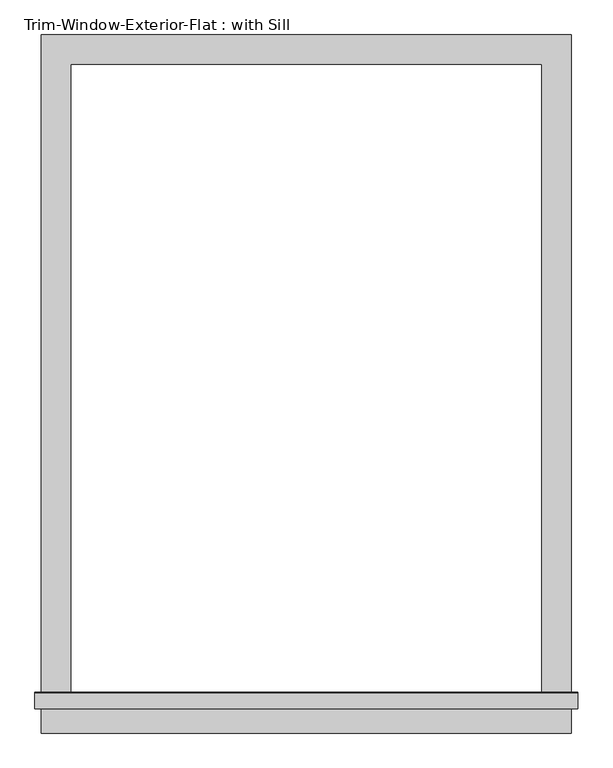
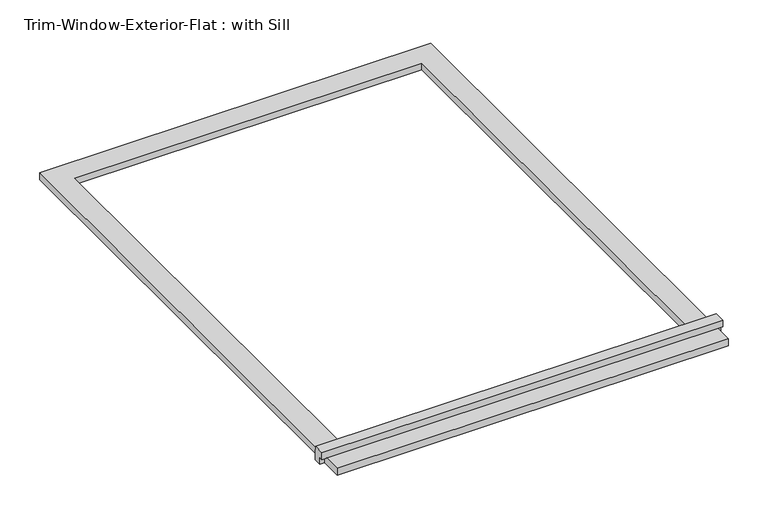
"""IFC4 building model written with IfcOpenShell, lengths in millimetres: proxy geometry, Trim-Window-Exterior-Flat : with Sill."""

from ifc_helpers import new_model, si_unit, frame, origin, origin_with_axes, place, context, project, spatial, polyline, outline, extrude, source, transform, mapped, element, save


def trim_window_exterior_flat_with_sill_e4b28ec3(model_context):
    return source(origin(), model_context, "Body", "SweptSolid", [
        extrude(outline(polyline([(514.35, -1241.3823709), (514.35, -1298.5323709), (-514.35, -1298.5323709), (-514.35, -1241.3823709), (514.35, -1241.3823709)])), origin_with_axes(), (0.0, 0.0, 1.0), 19.05),
        extrude(outline(polyline([(-1250.95, 38.1), (-1221.6580645, 38.1), (-1219.2, 19.05), (-1219.2, 0.0), (-1241.3823709, 0.0), (-1241.3823709, 19.05), (-1250.95, 19.05), (-1250.95, 38.1)])), frame((-527.05, 0.0, 0.0), z_axis=(1.0, 0.0, 0.0), x_axis=(0.0, 1.0, 0.0)), (0.0, 0.0, 1.0), 1054.1),
        extrude(outline(polyline([(-514.35, 57.15), (514.35, 57.15), (514.35, -1219.2), (457.2, -1219.2), (457.2, 0.0), (-457.2, 0.0), (-457.2, -1219.2), (-514.35, -1219.2), (-514.35, 57.15)])), origin_with_axes(), (0.0, 0.0, 1.0), 19.05),
    ])


if __name__ == "__main__":
    model = new_model("IFC4")
    model_context = context("Model", 3, world=origin())
    ifc_project = project(units=[si_unit("LENGTHUNIT", "METRE", prefix="MILLI")], contexts=[model_context])
    site = spatial("IfcSite", under=ifc_project)
    building = spatial("IfcBuilding", under=site)
    placement = place(None, origin())
    trim_window_exterior_flat_with_sill_shape = trim_window_exterior_flat_with_sill_e4b28ec3(model_context)
    element("IfcBuildingElementProxy", 1, Name="Trim-Window-Exterior-Flat : with Sill", ObjectType="Trim-Window-Exterior-Flat : with Sill", at=placement, inside=building, context=model_context, shape_type="MappedRepresentation", body=[
        mapped(trim_window_exterior_flat_with_sill_shape, transform((0.0, 0.0, 0.0), x_axis=(1.0, 0.0, 0.0), y_axis=(0.0, 1.0, 0.0), z_axis=(0.0, 0.0, 1.0))),
    ])
    save(model, "model.ifc")

# Revit data of these elements
# Type "Trim-Window-Exterior-Flat : with Sill"
#   Trim Width = 0' - 2 1/4"
#   Trim Thickness_Picture Frame = 0' - 1 1/4"
#   Trim Thickness_with Sill = 0' - 0 3/4"
#   Sill Thickness = 0' - 1 1/4"
#   Opening Width [instance default] = 2' - 0"
#   Opening Height [instance default] = 3' - 0"
#   Default Elevation = 4' - 0"
#   Sill = yes
#   Picture Frame = no
#   Trim Material [instance default] = none
# Element 1 (IfcBuildingElementProxy, "Trim-Window-Exterior-Flat : with Sill")
#   Opening Width = 3' - 0"
#   Opening Height = 4' - 0"
#   Trim Material = Clad - White
#   Materials on its faces: "Clad - White"
# Materials
#   "Clad - White": class "Wood", colour RGB 242 242 238, transparency 0, Cost = 0
